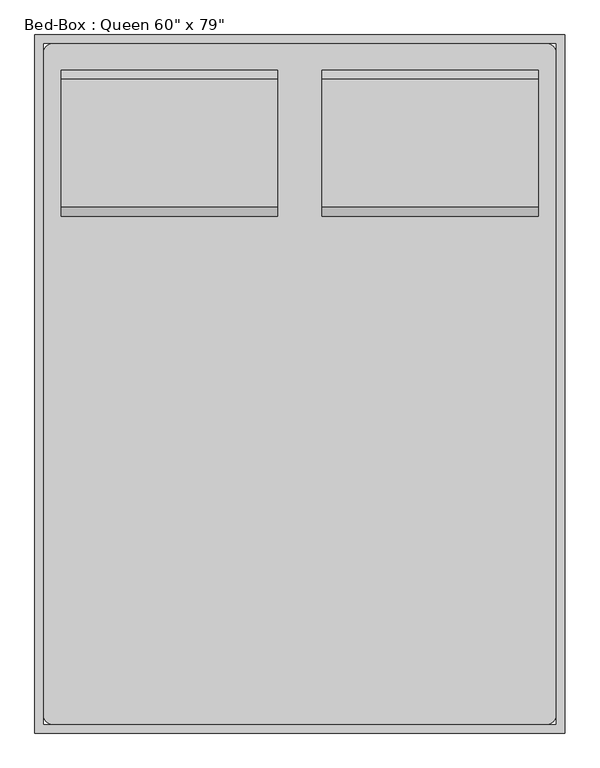
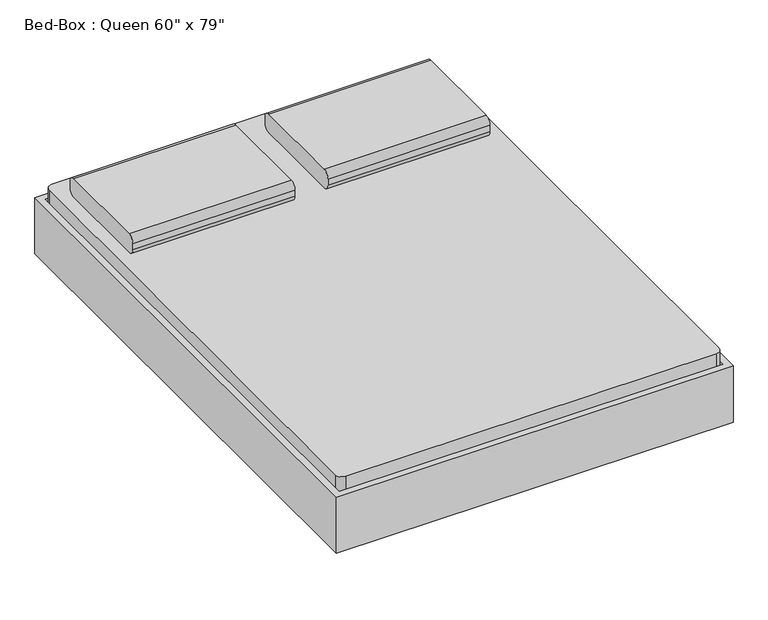
"""IFC4 building model written with IfcOpenShell, lengths in millimetres: furniture geometry."""

from ifc_helpers import new_model, si_unit, point, frame, frame_2d, origin, place, context, project, spatial, polyline, circle_curve, trimmed, segment, composite_curve, outline, extrude, source, transform, mapped, element, save
from ifc_brep_helpers import plane_surface, cylinder_surface, revolved_surface, advanced_brep


def furniture_1d2926bd(model_context):
    return source(origin(), model_context, "Body", "SolidModel", [
        extrude(outline(composite_curve([segment(polyline([(641.8704918, 406.4), (273.5704918, 406.4)]), True, "CONTINUOUS"), segment(trimmed(circle_curve(frame_2d((273.5704918, 431.8)), 25.4), [point((273.5704918, 406.4))], [point((248.1704918, 431.8))], False, "CARTESIAN"), True, "CONTINUOUS"), segment(polyline([(248.1704918, 431.8), (248.1704918, 457.2)]), True, "CONTINUOUS"), segment(trimmed(circle_curve(frame_2d((273.5704918, 457.2)), 25.4), [point((248.1704918, 457.2))], [point((273.5704918, 482.6))], False, "CARTESIAN"), True, "CONTINUOUS"), segment(polyline([(273.5704918, 482.6), (641.8704918, 482.6)]), True, "CONTINUOUS"), segment(trimmed(circle_curve(frame_2d((641.8704918, 457.2)), 25.4), [point((641.8704918, 482.6))], [point((667.2704918, 457.2))], False, "CARTESIAN"), True, "CONTINUOUS"), segment(polyline([(667.2704918, 457.2), (667.2704918, 431.8)]), True, "CONTINUOUS"), segment(trimmed(circle_curve(frame_2d((641.8704918, 431.8)), 25.4), [point((667.2704918, 431.8))], [point((641.8704918, 406.4))], False, "CARTESIAN"), True, "CONTINUOUS")], self_intersect=False)), frame((402.652459, 0.0, 0.0), z_axis=(1.0, 0.0, 0.0), x_axis=(0.0, 1.0, 0.0)), (0.0, 0.0, 1.0), 622.3),
        extrude(outline(composite_curve([segment(polyline([(641.8704918, 406.4), (273.5704918, 406.4)]), True, "CONTINUOUS"), segment(trimmed(circle_curve(frame_2d((273.5704918, 431.8)), 25.4), [point((273.5704918, 406.4))], [point((248.1704918, 431.8))], False, "CARTESIAN"), True, "CONTINUOUS"), segment(polyline([(248.1704918, 431.8), (248.1704918, 457.2)]), True, "CONTINUOUS"), segment(trimmed(circle_curve(frame_2d((273.5704918, 457.2)), 25.4), [point((248.1704918, 457.2))], [point((273.5704918, 482.6))], False, "CARTESIAN"), True, "CONTINUOUS"), segment(polyline([(273.5704918, 482.6), (641.8704918, 482.6)]), True, "CONTINUOUS"), segment(trimmed(circle_curve(frame_2d((641.8704918, 457.2)), 25.4), [point((641.8704918, 482.6))], [point((667.2704918, 457.2))], False, "CARTESIAN"), True, "CONTINUOUS"), segment(polyline([(667.2704918, 457.2), (667.2704918, 431.8)]), True, "CONTINUOUS"), segment(trimmed(circle_curve(frame_2d((641.8704918, 431.8)), 25.4), [point((667.2704918, 431.8))], [point((641.8704918, 406.4))], False, "CARTESIAN"), True, "CONTINUOUS")], self_intersect=False)), frame((-346.647541, 0.0, 0.0), z_axis=(1.0, 0.0, 0.0), x_axis=(0.0, 1.0, 0.0)), (0.0, 0.0, 1.0), 622.3),
        advanced_brep(
        [(-397.1231784, 514.8704918, 177.8), (-397.1231784, 438.6704918, 177.8), (-397.1231784, 438.6704918, 196.85), (-397.1231784, 514.8704918, 196.85), (-346.3231784, 514.8704918, 177.8), (-346.3231784, 438.6704918, 177.8), (-334.1869899, 438.6704918, 196.85), (-334.1869899, 514.8704918, 196.85), (-270.2523099, 514.8704918, 14.6654962), (-270.2523099, 438.6704918, 14.6654962), (-252.9871466, 438.6704918, 22.716374), (-252.9871466, 514.8704918, 22.716374), (-247.2320921, 438.6704918, 0.0), (-247.2320921, 514.8704918, 0.0), (-247.2320921, 438.6704918, 19.05), (-247.2320921, 514.8704918, 19.05), (-168.6195862, 514.8704918, 0.0), (-168.6195862, 438.6704918, 0.0), (-168.6195862, 438.6704918, 19.05), (-168.6195862, 514.8704918, 19.05), (-155.9195862, 438.6704918, 3.4029547), (-155.9195862, 514.8704918, 3.4029547), (-165.4445862, 438.6704918, 19.9007387), (-165.4445862, 514.8704918, 19.9007387), (-95.822541, 514.8704918, 38.1), (-95.822541, 438.6704918, 38.1), (-100.9269731, 438.6704918, 57.15), (-100.9269731, 514.8704918, 57.15), (774.4518216, 514.8704918, 38.1), (774.4518216, 438.6704918, 38.1), (779.5562537, 438.6704918, 57.15), (779.5562537, 514.8704918, 57.15), (834.5488669, 514.8704918, 3.4029547), (834.5488669, 438.6704918, 3.4029547), (844.0738669, 438.6704918, 19.9007387), (844.0738669, 514.8704918, 19.9007387), (847.2488669, 438.6704918, 0.0), (847.2488669, 514.8704918, 0.0), (847.2488669, 438.6704918, 19.05), (847.2488669, 514.8704918, 19.05), (925.8613728, 514.8704918, 0.0), (925.8613728, 438.6704918, 0.0), (925.8613728, 438.6704918, 19.05), (925.8613728, 514.8704918, 19.05), (948.8815906, 438.6704918, 14.6654962), (948.8815906, 514.8704918, 14.6654962), (931.6164272, 438.6704918, 22.716374), (931.6164272, 514.8704918, 22.716374), (1024.952459, 514.8704918, 177.8), (1024.952459, 438.6704918, 177.8), (1012.8162705, 438.6704918, 196.85), (1012.8162705, 514.8704918, 196.85), (1075.752459, 514.8704918, 177.8), (1075.752459, 514.8704918, 196.85), (1075.752459, 438.6704918, 196.85), (1075.752459, 438.6704918, 177.8)],
        [
            (0, 1),
            (1, 2),
            (2, 3),
            (3, 0),
            (0, 4),
            (4, 5),
            (5, 1),
            (5, 6),
            (6, 2),
            (6, 7),
            (7, 3),
            (7, 4),
            (4, 8),
            (8, 9),
            (9, 5),
            (9, 10),
            (10, 6),
            (10, 11),
            (11, 7),
            (11, 8),
            (12, 9, circle_curve(frame((-247.2320921, 438.6704918, 25.4), z_axis=(0.0, 1.0, 0.0), x_axis=(-0.9063077870366486, 0.0, -0.42261826174070233)), 25.4)),
            (8, 13, circle_curve(frame((-247.2320921, 514.8704918, 25.4), z_axis=(0.0, -1.0, 0.0), x_axis=(-0.9063077870366486, 0.0, -0.42261826174070233)), 25.4)),
            (13, 12),
            (14, 10, circle_curve(frame((-247.2320921, 438.6704918, 25.4), z_axis=(0.0, 1.0, 0.0), x_axis=(-0.9063077870366486, 0.0, -0.42261826174070233)), 6.35)),
            (12, 14),
            (15, 11, circle_curve(frame((-247.2320921, 514.8704918, 25.4), z_axis=(0.0, 1.0, 0.0), x_axis=(-0.9063077870366486, 0.0, -0.42261826174070233)), 6.35)),
            (14, 15),
            (15, 13),
            (13, 16),
            (16, 17),
            (17, 12),
            (17, 18),
            (18, 14),
            (18, 19),
            (19, 15),
            (19, 16),
            (20, 17, circle_curve(frame((-168.6195862, 438.6704918, 25.4), z_axis=(0.0, 1.0, 0.0), x_axis=(0.0, 0.0, -1.0)), 25.4)),
            (16, 21, circle_curve(frame((-168.6195862, 514.8704918, 25.4), z_axis=(0.0, -1.0, 0.0), x_axis=(0.0, 0.0, -1.0)), 25.4)),
            (21, 20),
            (22, 18, circle_curve(frame((-168.6195862, 438.6704918, 25.4), z_axis=(0.0, 1.0, 0.0), x_axis=(0.0, 0.0, -1.0)), 6.35)),
            (20, 22),
            (23, 19, circle_curve(frame((-168.6195862, 514.8704918, 25.4), z_axis=(0.0, 1.0, 0.0), x_axis=(0.0, 0.0, -1.0)), 6.35)),
            (22, 23),
            (23, 21),
            (21, 24),
            (24, 25),
            (25, 20),
            (25, 26),
            (26, 22),
            (26, 27),
            (27, 23),
            (27, 24),
            (24, 28),
            (28, 29),
            (29, 25),
            (29, 30),
            (30, 26),
            (30, 31),
            (31, 27),
            (31, 28),
            (28, 32),
            (32, 33),
            (33, 29),
            (33, 34),
            (34, 30),
            (34, 35),
            (35, 31),
            (35, 32),
            (36, 33, circle_curve(frame((847.2488669, 438.6704918, 25.4), z_axis=(0.0, 1.0, 0.0), x_axis=(-0.5000000000000463, 0.0, -0.8660254037844118)), 25.4)),
            (32, 37, circle_curve(frame((847.2488669, 514.8704918, 25.4), z_axis=(0.0, -1.0, 0.0), x_axis=(-0.5000000000000463, 0.0, -0.8660254037844118)), 25.4)),
            (37, 36),
            (38, 34, circle_curve(frame((847.2488669, 438.6704918, 25.4), z_axis=(0.0, 1.0, 0.0), x_axis=(-0.5000000000000463, 0.0, -0.8660254037844118)), 6.35)),
            (36, 38),
            (39, 35, circle_curve(frame((847.2488669, 514.8704918, 25.4), z_axis=(0.0, 1.0, 0.0), x_axis=(-0.5000000000000463, 0.0, -0.8660254037844118)), 6.35)),
            (38, 39),
            (39, 37),
            (37, 40),
            (40, 41),
            (41, 36),
            (41, 42),
            (42, 38),
            (42, 43),
            (43, 39),
            (43, 40),
            (44, 41, circle_curve(frame((925.8613728, 438.6704918, 25.4), z_axis=(0.0, 1.0, 0.0), x_axis=(0.0, 0.0, -1.0)), 25.4)),
            (40, 45, circle_curve(frame((925.8613728, 514.8704918, 25.4), z_axis=(0.0, -1.0, 0.0), x_axis=(0.0, 0.0, -1.0)), 25.4)),
            (45, 44),
            (46, 42, circle_curve(frame((925.8613728, 438.6704918, 25.4), z_axis=(0.0, 1.0, 0.0), x_axis=(0.0, 0.0, -1.0)), 6.35)),
            (44, 46),
            (47, 43, circle_curve(frame((925.8613728, 514.8704918, 25.4), z_axis=(0.0, 1.0, 0.0), x_axis=(0.0, 0.0, -1.0)), 6.35)),
            (46, 47),
            (47, 45),
            (45, 48),
            (48, 49),
            (49, 44),
            (49, 50),
            (50, 46),
            (50, 51),
            (51, 47),
            (51, 48),
            (52, 53),
            (53, 54),
            (54, 55),
            (55, 52),
            (48, 52),
            (55, 49),
            (54, 50),
            (53, 51),
        ],
        [
            plane_surface(frame((-397.1231784, 768.8704918, -152.9490627), z_axis=(-1.0, 0.0, 0.0), x_axis=(0.0, 1.0, 0.0))),
            plane_surface(frame((-397.1231784, 514.8704918, 177.8), z_axis=(0.0, 0.0, -1.0), x_axis=(1.0, 0.0, 0.0))),
            plane_surface(frame((-397.1231784, 438.6704918, 177.8), z_axis=(0.0, -1.0, 0.0), x_axis=(1.0, 0.0, 0.0))),
            plane_surface(frame((-397.1231784, 438.6704918, 196.85), z_axis=(0.0, 0.0, 1.0), x_axis=(1.0, 0.0, 0.0))),
            plane_surface(frame((-397.1231784, 514.8704918, 196.85), z_axis=(0.0, 1.0, 0.0), x_axis=(1.0, 0.0, 0.0))),
            plane_surface(frame((-346.3231784, 514.8704918, 177.8), z_axis=(-0.9063077870366485, 0.0, -0.4226182617407027), x_axis=(0.4226182617407027, 0.0, -0.9063077870366485))),
            plane_surface(frame((-346.3231784, 438.6704918, 177.8), z_axis=(0.0, -1.0, 0.0), x_axis=(0.4226182617407025, 0.0, -0.9063077870366486))),
            plane_surface(frame((-334.1869899, 438.6704918, 196.85), z_axis=(0.9063077870366484, 0.0, 0.4226182617407028), x_axis=(0.4226182617407028, 0.0, -0.9063077870366484))),
            plane_surface(frame((-334.1869899, 514.8704918, 196.85), z_axis=(0.0, 1.0, 0.0), x_axis=(0.42261826174070277, 0.0, -0.9063077870366485))),
            cylinder_surface(frame((-247.2320921, 768.8704918, 25.4), z_axis=(0.0, -1.0, 0.0), x_axis=(-0.9063077870366486, 0.0, -0.42261826174070233)), 25.4),
            plane_surface(frame((-247.2320921, 438.6704918, 25.4), z_axis=(0.0, -1.0, 0.0), x_axis=(-0.9063077870366486, 0.0, -0.42261826174070233))),
            revolved_surface(polyline([(-252.9871465476827, 438.6704918, 22.71637403794654), (-252.9871465476827, 514.8704918, 22.71637403794654)]), (-247.2320921, 768.8704918, 25.4), (0.0, -1.0, 0.0)),
            plane_surface(frame((-247.2320921, 514.8704918, 25.4), z_axis=(0.0, 1.0, 0.0), x_axis=(-0.9063077870366486, 0.0, -0.42261826174070233))),
            plane_surface(frame((-247.2320921, 514.8704918, 0.0), z_axis=(0.0, 0.0, -1.0), x_axis=(1.0, 0.0, 0.0))),
            plane_surface(frame((-247.2320921, 438.6704918, 0.0), z_axis=(0.0, -1.0, 0.0), x_axis=(1.0, 0.0, 0.0))),
            plane_surface(frame((-247.2320921, 438.6704918, 19.05), z_axis=(0.0, 0.0, 1.0), x_axis=(1.0, 0.0, 0.0))),
            plane_surface(frame((-247.2320921, 514.8704918, 19.05), z_axis=(0.0, 1.0, 0.0), x_axis=(1.0, 0.0, 0.0))),
            cylinder_surface(frame((-168.6195862, 768.8704918, 25.4), z_axis=(0.0, -1.0, 0.0), x_axis=(0.0, 0.0, -1.0)), 25.4),
            plane_surface(frame((-168.6195862, 438.6704918, 25.4), z_axis=(0.0, -1.0, 0.0), x_axis=(0.0, 0.0, -1.0))),
            revolved_surface(polyline([(-168.6195862, 438.6704918, 19.049999999999997), (-168.6195862, 514.8704918, 19.049999999999997)]), (-168.6195862, 768.8704918, 25.4), (0.0, -1.0, 0.0)),
            plane_surface(frame((-168.6195862, 514.8704918, 25.4), z_axis=(0.0, 1.0, 0.0), x_axis=(0.0, 0.0, -1.0))),
            plane_surface(frame((-155.9195862, 514.8704918, 3.4029547), z_axis=(0.49999999999988004, 0.0, -0.866025403784508), x_axis=(0.866025403784508, 0.0, 0.49999999999988004))),
            plane_surface(frame((-155.9195862, 438.6704918, 3.4029547), z_axis=(0.0, -1.0, 0.0), x_axis=(0.8660254037845078, 0.0, 0.49999999999988026))),
            plane_surface(frame((-165.4445862, 438.6704918, 19.9007387), z_axis=(-0.4999999999998799, 0.0, 0.866025403784508), x_axis=(0.866025403784508, 0.0, 0.4999999999998799))),
            plane_surface(frame((-165.4445862, 514.8704918, 19.9007387), z_axis=(0.0, 1.0, 0.0), x_axis=(0.8660254037845075, 0.0, 0.49999999999988076))),
            plane_surface(frame((-95.822541, 514.8704918, 38.1), z_axis=(0.0, 0.0, -1.0), x_axis=(1.0, 0.0, 0.0))),
            plane_surface(frame((-95.822541, 438.6704918, 38.1), z_axis=(0.0, -1.0, 0.0), x_axis=(1.0, 0.0, 0.0))),
            plane_surface(frame((-100.9269731, 438.6704918, 57.15), z_axis=(0.0, 0.0, 1.0), x_axis=(1.0, 0.0, 0.0))),
            plane_surface(frame((-100.9269731, 514.8704918, 57.15), z_axis=(0.0, 1.0, 0.0), x_axis=(1.0, 0.0, 0.0))),
            plane_surface(frame((774.4518216, 514.8704918, 38.1), z_axis=(-0.5000000000000455, 0.0, -0.8660254037844125), x_axis=(0.8660254037844125, 0.0, -0.5000000000000455))),
            plane_surface(frame((774.4518216, 438.6704918, 38.1), z_axis=(0.0, -1.0, 0.0), x_axis=(0.866025403784412, 0.0, -0.5000000000000463))),
            plane_surface(frame((779.5562537, 438.6704918, 57.15), z_axis=(0.5000000000000466, 0.0, 0.8660254037844117), x_axis=(0.8660254037844117, 0.0, -0.5000000000000466))),
            plane_surface(frame((779.5562537, 514.8704918, 57.15), z_axis=(0.0, 1.0, 0.0), x_axis=(0.8660254037844115, 0.0, -0.5000000000000471))),
            cylinder_surface(frame((847.2488669, 768.8704918, 25.4), z_axis=(0.0, -1.0, 0.0), x_axis=(-0.5000000000000463, 0.0, -0.8660254037844118)), 25.4),
            plane_surface(frame((847.2488669, 438.6704918, 25.4), z_axis=(0.0, -1.0000000000000002, 0.0), x_axis=(-0.5000000000000464, 0.0, -0.866025403784412))),
            revolved_surface(polyline([(844.0738668999998, 438.6704918, 19.90073868596898), (844.0738668999998, 514.8704918, 19.90073868596898)]), (847.2488669, 768.8704918, 25.4), (0.0, -1.0, 0.0)),
            plane_surface(frame((847.2488669, 514.8704918, 25.4), z_axis=(0.0, 1.0000000000000002, 0.0), x_axis=(-0.5000000000000464, 0.0, -0.866025403784412))),
            plane_surface(frame((847.2488669, 514.8704918, 0.0), z_axis=(0.0, 0.0, -1.0), x_axis=(1.0, 0.0, 0.0))),
            plane_surface(frame((847.2488669, 438.6704918, 0.0), z_axis=(0.0, -1.0, 0.0), x_axis=(1.0, 0.0, 0.0))),
            plane_surface(frame((847.2488669, 438.6704918, 19.05), z_axis=(0.0, 0.0, 1.0), x_axis=(1.0, 0.0, 0.0))),
            plane_surface(frame((847.2488669, 514.8704918, 19.05), z_axis=(0.0, 1.0, 0.0), x_axis=(1.0, 0.0, 0.0))),
            cylinder_surface(frame((925.8613728, 768.8704918, 25.4), z_axis=(0.0, -1.0, 0.0), x_axis=(0.0, 0.0, -1.0)), 25.4),
            plane_surface(frame((925.8613728, 438.6704918, 25.4), z_axis=(0.0, -1.0, 0.0), x_axis=(0.0, 0.0, -1.0))),
            revolved_surface(polyline([(925.8613728, 438.6704918, 19.049999999999997), (925.8613728, 514.8704918, 19.049999999999997)]), (925.8613728, 768.8704918, 25.4), (0.0, -1.0, 0.0)),
            plane_surface(frame((925.8613728, 514.8704918, 25.4), z_axis=(0.0, 1.0, 0.0), x_axis=(0.0, 0.0, -1.0))),
            plane_surface(frame((948.8815906, 514.8704918, 14.6654962), z_axis=(0.90630778703668, 0.0, -0.42261826174063505), x_axis=(0.42261826174063505, 0.0, 0.90630778703668))),
            plane_surface(frame((948.8815906, 438.6704918, 14.6654962), z_axis=(0.0, -1.0, 0.0), x_axis=(0.42261826174063566, 0.0, 0.9063077870366797))),
            plane_surface(frame((931.6164272, 438.6704918, 22.716374), z_axis=(-0.9063077870366801, 0.0, 0.42261826174063477), x_axis=(0.42261826174063477, 0.0, 0.9063077870366801))),
            plane_surface(frame((931.6164272, 514.8704918, 22.716374), z_axis=(0.0, 1.0, 0.0), x_axis=(0.4226182617406345, 0.0, 0.9063077870366802))),
            plane_surface(frame((1075.752459, 768.8704918, -152.9490627), z_axis=(1.0, 0.0, 0.0), x_axis=(0.0, 1.0, 0.0))),
            plane_surface(frame((1024.952459, 514.8704918, 177.8), z_axis=(0.0, 0.0, -1.0), x_axis=(1.0, 0.0, 0.0))),
            plane_surface(frame((1024.952459, 438.6704918, 177.8), z_axis=(0.0, -1.0, 0.0), x_axis=(1.0, 0.0, 0.0))),
            plane_surface(frame((1012.8162705, 438.6704918, 196.85), z_axis=(0.0, 0.0, 1.0), x_axis=(1.0, 0.0, 0.0))),
            plane_surface(frame((1012.8162705, 514.8704918, 196.85), z_axis=(0.0, 1.0, 0.0), x_axis=(1.0, 0.0, 0.0))),
        ],
        [
            (0, [[1, 2, 3, 4]]),
            (1, [[-1, 5, 6, 7]]),
            (2, [[-2, -7, 8, 9]]),
            (3, [[-3, -9, 10, 11]]),
            (4, [[-4, -11, 12, -5]]),
            (5, [[-6, 13, 14, 15]]),
            (6, [[-8, -15, 16, 17]]),
            (7, [[-10, -17, 18, 19]]),
            (8, [[-12, -19, 20, -13]]),
            (9, [[21, -14, 22, 23]]),
            (10, [[24, -16, -21, 25]]),
            (11, [[26, -18, -24, 27]]),
            (12, [[-22, -20, -26, 28]]),
            (13, [[-23, 29, 30, 31]]),
            (14, [[-25, -31, 32, 33]]),
            (15, [[-27, -33, 34, 35]]),
            (16, [[-28, -35, 36, -29]]),
            (17, [[37, -30, 38, 39]]),
            (18, [[40, -32, -37, 41]]),
            (19, [[42, -34, -40, 43]]),
            (20, [[-38, -36, -42, 44]]),
            (21, [[-39, 45, 46, 47]]),
            (22, [[-41, -47, 48, 49]]),
            (23, [[-43, -49, 50, 51]]),
            (24, [[-44, -51, 52, -45]]),
            (25, [[-46, 53, 54, 55]]),
            (26, [[-48, -55, 56, 57]]),
            (27, [[-50, -57, 58, 59]]),
            (28, [[-52, -59, 60, -53]]),
            (29, [[-54, 61, 62, 63]]),
            (30, [[-56, -63, 64, 65]]),
            (31, [[-58, -65, 66, 67]]),
            (32, [[-60, -67, 68, -61]]),
            (33, [[69, -62, 70, 71]]),
            (34, [[72, -64, -69, 73]]),
            (35, [[74, -66, -72, 75]]),
            (36, [[-70, -68, -74, 76]]),
            (37, [[-71, 77, 78, 79]]),
            (38, [[-73, -79, 80, 81]]),
            (39, [[-75, -81, 82, 83]]),
            (40, [[-76, -83, 84, -77]]),
            (41, [[85, -78, 86, 87]]),
            (42, [[88, -80, -85, 89]]),
            (43, [[90, -82, -88, 91]]),
            (44, [[-86, -84, -90, 92]]),
            (45, [[-87, 93, 94, 95]]),
            (46, [[-89, -95, 96, 97]]),
            (47, [[-91, -97, 98, 99]]),
            (48, [[-92, -99, 100, -93]]),
            (49, [[101, 102, 103, 104]]),
            (50, [[-94, 105, -104, 106]]),
            (51, [[-96, -106, -103, 107]]),
            (52, [[-98, -107, -102, 108]]),
            (53, [[-100, -108, -101, -105]]),
        ],
    ),
        extrude(outline(composite_curve([segment(polyline([(-372.047541, 743.4704918), (1050.352459, 743.4704918)]), True, "CONTINUOUS"), segment(trimmed(circle_curve(frame_2d((1050.352459, 718.0704918)), 25.4), [point((1050.352459, 743.4704918))], [point((1075.752459, 718.0704918))], False, "CARTESIAN"), True, "CONTINUOUS"), segment(polyline([(1075.752459, 718.0704918), (1075.752459, -1186.9295082)]), True, "CONTINUOUS"), segment(trimmed(circle_curve(frame_2d((1050.352459, -1186.9295082)), 25.4), [point((1075.752459, -1186.9295082))], [point((1050.352459, -1212.3295082))], False, "CARTESIAN"), True, "CONTINUOUS"), segment(polyline([(1050.352459, -1212.3295082), (-372.047541, -1212.3295082)]), True, "CONTINUOUS"), segment(trimmed(circle_curve(frame_2d((-372.047541, -1186.9295082)), 25.4), [point((-372.047541, -1212.3295082))], [point((-397.447541, -1186.9295082))], False, "CARTESIAN"), True, "CONTINUOUS"), segment(polyline([(-397.447541, -1186.9295082), (-397.447541, 718.0704918)]), True, "CONTINUOUS"), segment(trimmed(circle_curve(frame_2d((-372.047541, 718.0704918)), 25.4), [point((-397.447541, 718.0704918))], [point((-372.047541, 743.4704918))], False, "CARTESIAN"), True, "CONTINUOUS")], self_intersect=False)), frame((0.0, 0.0, 203.2), z_axis=(0.0, 0.0, 1.0), x_axis=(1.0, 0.0, 0.0)), (0.0, 0.0, 1.0), 203.2),
        advanced_brep(
        [(-397.447541, -932.9295082, 196.85), (-397.447541, -932.9295082, 177.8), (-397.447541, -1009.1295082, 177.8), (-397.447541, -1009.1295082, 196.85), (-334.5113525, -932.9295082, 196.85), (-346.647541, -932.9295082, 177.8), (-346.647541, -1009.1295082, 177.8), (-334.5113525, -1009.1295082, 196.85), (-253.3115092, -932.9295082, 22.716374), (-270.5766725, -932.9295082, 14.6654962), (-270.5766725, -1009.1295082, 14.6654962), (-253.3115092, -1009.1295082, 22.716374), (-247.5564547, -932.9295082, 0.0), (-247.5564547, -932.9295082, 19.05), (-247.5564547, -1009.1295082, 0.0), (-247.5564547, -1009.1295082, 19.05), (-168.9439489, -932.9295082, 19.05), (-168.9439489, -932.9295082, 0.0), (-168.9439489, -1009.1295082, 0.0), (-168.9439489, -1009.1295082, 19.05), (-156.2439489, -932.9295082, 3.4029547), (-165.7689489, -932.9295082, 19.9007387), (-156.2439489, -1009.1295082, 3.4029547), (-165.7689489, -1009.1295082, 19.9007387), (-101.2513357, -932.9295082, 57.15), (-96.1469036, -932.9295082, 38.1), (-96.1469036, -1009.1295082, 38.1), (-101.2513357, -1009.1295082, 57.15), (779.5562537, -932.9295082, 57.15), (774.4518216, -932.9295082, 38.1), (774.4518216, -1009.1295082, 38.1), (779.5562537, -1009.1295082, 57.15), (844.0738669, -932.9295082, 19.9007387), (834.5488669, -932.9295082, 3.4029547), (834.5488669, -1009.1295082, 3.4029547), (844.0738669, -1009.1295082, 19.9007387), (847.2488669, -932.9295082, 0.0), (847.2488669, -932.9295082, 19.05), (847.2488669, -1009.1295082, 0.0), (847.2488669, -1009.1295082, 19.05), (925.8613728, -932.9295082, 19.05), (925.8613728, -932.9295082, 0.0), (925.8613728, -1009.1295082, 0.0), (925.8613728, -1009.1295082, 19.05), (948.8815906, -932.9295082, 14.6654962), (931.6164272, -932.9295082, 22.716374), (948.8815906, -1009.1295082, 14.6654962), (931.6164272, -1009.1295082, 22.716374), (1012.8162705, -932.9295082, 196.85), (1024.952459, -932.9295082, 177.8), (1024.952459, -1009.1295082, 177.8), (1012.8162705, -1009.1295082, 196.85), (1075.752459, -932.9295082, 196.85), (1075.752459, -1009.1295082, 196.85), (1075.752459, -1009.1295082, 177.8), (1075.752459, -932.9295082, 177.8)],
        [
            (0, 1),
            (1, 2),
            (2, 3),
            (3, 0),
            (0, 4),
            (4, 5),
            (5, 1),
            (5, 6),
            (6, 2),
            (6, 7),
            (7, 3),
            (7, 4),
            (4, 8),
            (8, 9),
            (9, 5),
            (9, 10),
            (10, 6),
            (10, 11),
            (11, 7),
            (11, 8),
            (12, 9, circle_curve(frame((-247.5564547, -932.9295082, 25.4), z_axis=(0.0, 1.0, 0.0), x_axis=(-0.906307787036663, 0.0, -0.4226182617406713)), 25.4)),
            (8, 13, circle_curve(frame((-247.5564547, -932.9295082, 25.4), z_axis=(0.0, -1.0, 0.0), x_axis=(-0.906307787036663, 0.0, -0.4226182617406713)), 6.35)),
            (13, 12),
            (14, 10, circle_curve(frame((-247.5564547, -1009.1295082, 25.4), z_axis=(0.0, 1.0, 0.0), x_axis=(-0.906307787036663, 0.0, -0.4226182617406713)), 25.4)),
            (12, 14),
            (15, 11, circle_curve(frame((-247.5564547, -1009.1295082, 25.4), z_axis=(0.0, 1.0, 0.0), x_axis=(-0.906307787036663, 0.0, -0.4226182617406713)), 6.35)),
            (14, 15),
            (15, 13),
            (13, 16),
            (16, 17),
            (17, 12),
            (17, 18),
            (18, 14),
            (18, 19),
            (19, 15),
            (19, 16),
            (20, 17, circle_curve(frame((-168.9439489, -932.9295082, 25.4), z_axis=(0.0, 1.0, 0.0), x_axis=(0.0, 0.0, -1.0)), 25.4)),
            (16, 21, circle_curve(frame((-168.9439489, -932.9295082, 25.4), z_axis=(0.0, -1.0, 0.0), x_axis=(0.0, 0.0, -1.0)), 6.35)),
            (21, 20),
            (22, 18, circle_curve(frame((-168.9439489, -1009.1295082, 25.4), z_axis=(0.0, 1.0, 0.0), x_axis=(0.0, 0.0, -1.0)), 25.4)),
            (20, 22),
            (23, 19, circle_curve(frame((-168.9439489, -1009.1295082, 25.4), z_axis=(0.0, 1.0, 0.0), x_axis=(0.0, 0.0, -1.0)), 6.35)),
            (22, 23),
            (23, 21),
            (21, 24),
            (24, 25),
            (25, 20),
            (25, 26),
            (26, 22),
            (26, 27),
            (27, 23),
            (27, 24),
            (24, 28),
            (28, 29),
            (29, 25),
            (29, 30),
            (30, 26),
            (30, 31),
            (31, 27),
            (31, 28),
            (28, 32),
            (32, 33),
            (33, 29),
            (33, 34),
            (34, 30),
            (34, 35),
            (35, 31),
            (35, 32),
            (36, 33, circle_curve(frame((847.2488669, -932.9295082, 25.4), z_axis=(0.0, 1.0, 0.0), x_axis=(-0.5000000000000479, 0.0, -0.866025403784411)), 25.4)),
            (32, 37, circle_curve(frame((847.2488669, -932.9295082, 25.4), z_axis=(0.0, -1.0, 0.0), x_axis=(-0.5000000000000479, 0.0, -0.866025403784411)), 6.35)),
            (37, 36),
            (38, 34, circle_curve(frame((847.2488669, -1009.1295082, 25.4), z_axis=(0.0, 1.0, 0.0), x_axis=(-0.5000000000000479, 0.0, -0.866025403784411)), 25.4)),
            (36, 38),
            (39, 35, circle_curve(frame((847.2488669, -1009.1295082, 25.4), z_axis=(0.0, 1.0, 0.0), x_axis=(-0.5000000000000479, 0.0, -0.866025403784411)), 6.35)),
            (38, 39),
            (39, 37),
            (37, 40),
            (40, 41),
            (41, 36),
            (41, 42),
            (42, 38),
            (42, 43),
            (43, 39),
            (43, 40),
            (44, 41, circle_curve(frame((925.8613728, -932.9295082, 25.4), z_axis=(0.0, 1.0, 0.0), x_axis=(0.0, 0.0, -1.0)), 25.4)),
            (40, 45, circle_curve(frame((925.8613728, -932.9295082, 25.4), z_axis=(0.0, -1.0, 0.0), x_axis=(0.0, 0.0, -1.0)), 6.35)),
            (45, 44),
            (46, 42, circle_curve(frame((925.8613728, -1009.1295082, 25.4), z_axis=(0.0, 1.0, 0.0), x_axis=(0.0, 0.0, -1.0)), 25.4)),
            (44, 46),
            (47, 43, circle_curve(frame((925.8613728, -1009.1295082, 25.4), z_axis=(0.0, 1.0, 0.0), x_axis=(0.0, 0.0, -1.0)), 6.35)),
            (46, 47),
            (47, 45),
            (45, 48),
            (48, 49),
            (49, 44),
            (49, 50),
            (50, 46),
            (50, 51),
            (51, 47),
            (51, 48),
            (52, 53),
            (53, 54),
            (54, 55),
            (55, 52),
            (48, 52),
            (55, 49),
            (54, 50),
            (53, 51),
        ],
        [
            plane_surface(frame((-397.447541, -1237.7295082, -127.5947323), z_axis=(-1.0, 0.0, 0.0), x_axis=(0.0, 1.0, 0.0))),
            plane_surface(frame((-397.447541, -932.9295082, 196.85), z_axis=(0.0, 1.0, 0.0), x_axis=(1.0, 0.0, 0.0))),
            plane_surface(frame((-397.447541, -932.9295082, 177.8), z_axis=(0.0, 0.0, -1.0), x_axis=(1.0, 0.0, 0.0))),
            plane_surface(frame((-397.447541, -1009.1295082, 177.8), z_axis=(0.0, -1.0, 0.0), x_axis=(1.0, 0.0, 0.0))),
            plane_surface(frame((-397.447541, -1009.1295082, 196.85), z_axis=(0.0, 0.0, 1.0), x_axis=(1.0, 0.0, 0.0))),
            plane_surface(frame((-334.5113525, -932.9295082, 196.85), z_axis=(0.0, 1.0, 0.0), x_axis=(0.4226182617406707, 0.0, -0.9063077870366634))),
            plane_surface(frame((-346.647541, -932.9295082, 177.8), z_axis=(-0.9063077870366635, 0.0, -0.4226182617406707), x_axis=(0.4226182617406707, 0.0, -0.9063077870366635))),
            plane_surface(frame((-346.647541, -1009.1295082, 177.8), z_axis=(0.0, -1.0, 0.0), x_axis=(0.422618261740671, 0.0, -0.9063077870366633))),
            plane_surface(frame((-334.5113525, -1009.1295082, 196.85), z_axis=(0.9063077870366633, 0.0, 0.42261826174067113), x_axis=(0.42261826174067113, 0.0, -0.9063077870366633))),
            plane_surface(frame((-247.5564547, -932.9295082, 25.4), z_axis=(0.0, 1.0, 0.0), x_axis=(-0.906307787036663, 0.0, -0.4226182617406713))),
            cylinder_surface(frame((-247.5564547, -1237.7295082, 25.4), z_axis=(0.0, -1.0, 0.0), x_axis=(-0.906307787036663, 0.0, -0.4226182617406713)), 25.4),
            plane_surface(frame((-247.5564547, -1009.1295082, 25.4), z_axis=(0.0, -1.0, 0.0), x_axis=(-0.906307787036663, 0.0, -0.4226182617406713))),
            revolved_surface(polyline([(-253.3115091476828, -1009.1295082, 22.716374037946736), (-253.3115091476828, -932.9295082, 22.716374037946736)]), (-247.5564547, -1237.7295082, 25.4), (0.0, -1.0, 0.0)),
            plane_surface(frame((-247.5564547, -932.9295082, 19.05), z_axis=(0.0, 1.0, 0.0), x_axis=(1.0, 0.0, 0.0))),
            plane_surface(frame((-247.5564547, -932.9295082, 0.0), z_axis=(0.0, 0.0, -1.0), x_axis=(1.0, 0.0, 0.0))),
            plane_surface(frame((-247.5564547, -1009.1295082, 0.0), z_axis=(0.0, -1.0, 0.0), x_axis=(1.0, 0.0, 0.0))),
            plane_surface(frame((-247.5564547, -1009.1295082, 19.05), z_axis=(0.0, 0.0, 1.0), x_axis=(1.0, 0.0, 0.0))),
            plane_surface(frame((-168.9439489, -932.9295082, 25.4), z_axis=(0.0, 1.0, 0.0), x_axis=(0.0, 0.0, -1.0))),
            cylinder_surface(frame((-168.9439489, -1237.7295082, 25.4), z_axis=(0.0, -1.0, 0.0), x_axis=(0.0, 0.0, -1.0)), 25.4),
            plane_surface(frame((-168.9439489, -1009.1295082, 25.4), z_axis=(0.0, -1.0, 0.0), x_axis=(0.0, 0.0, -1.0))),
            revolved_surface(polyline([(-168.9439489, -1009.1295082, 19.049999999999997), (-168.9439489, -932.9295082, 19.049999999999997)]), (-168.9439489, -1237.7295082, 25.4), (0.0, -1.0, 0.0)),
            plane_surface(frame((-165.7689489, -932.9295082, 19.9007387), z_axis=(0.0, 1.0, 0.0), x_axis=(0.8660254037844788, 0.0, 0.4999999999999306))),
            plane_surface(frame((-156.2439489, -932.9295082, 3.4029547), z_axis=(0.49999999999993017, 0.0, -0.866025403784479), x_axis=(0.866025403784479, 0.0, 0.49999999999993017))),
            plane_surface(frame((-156.2439489, -1009.1295082, 3.4029547), z_axis=(0.0, -1.0, 0.0), x_axis=(0.8660254037844785, 0.0, 0.49999999999993106))),
            plane_surface(frame((-165.7689489, -1009.1295082, 19.9007387), z_axis=(-0.4999999999999309, 0.0, 0.8660254037844786), x_axis=(0.8660254037844786, 0.0, 0.4999999999999309))),
            plane_surface(frame((-101.2513357, -932.9295082, 57.15), z_axis=(0.0, 1.0, 0.0), x_axis=(1.0, 0.0, 0.0))),
            plane_surface(frame((-96.1469036, -932.9295082, 38.1), z_axis=(0.0, 0.0, -1.0), x_axis=(1.0, 0.0, 0.0))),
            plane_surface(frame((-96.1469036, -1009.1295082, 38.1), z_axis=(0.0, -1.0, 0.0), x_axis=(1.0, 0.0, 0.0))),
            plane_surface(frame((-101.2513357, -1009.1295082, 57.15), z_axis=(0.0, 0.0, 1.0), x_axis=(1.0, 0.0, 0.0))),
            plane_surface(frame((779.5562537, -932.9295082, 57.15), z_axis=(0.0, 1.0000000000000002, 0.0), x_axis=(0.8660254037844106, 0.0, -0.5000000000000487))),
            plane_surface(frame((774.4518216, -932.9295082, 38.1), z_axis=(-0.5000000000000477, 0.0, -0.8660254037844112), x_axis=(0.8660254037844112, 0.0, -0.5000000000000477))),
            plane_surface(frame((774.4518216, -1009.1295082, 38.1), z_axis=(0.0, -1.0000000000000002, 0.0), x_axis=(0.8660254037844105, 0.0, -0.500000000000049))),
            plane_surface(frame((779.5562537, -1009.1295082, 57.15), z_axis=(0.5000000000000498, 0.0, 0.8660254037844098), x_axis=(0.8660254037844098, 0.0, -0.5000000000000498))),
            plane_surface(frame((847.2488669, -932.9295082, 25.4), z_axis=(0.0, 1.0000000000000002, 0.0), x_axis=(-0.500000000000048, 0.0, -0.8660254037844111))),
            cylinder_surface(frame((847.2488669, -1237.7295082, 25.4), z_axis=(0.0, -1.0, 0.0), x_axis=(-0.5000000000000479, 0.0, -0.866025403784411)), 25.4),
            plane_surface(frame((847.2488669, -1009.1295082, 25.4), z_axis=(0.0, -1.0000000000000002, 0.0), x_axis=(-0.500000000000048, 0.0, -0.8660254037844111))),
            revolved_surface(polyline([(844.0738668999998, -1009.1295082, 19.90073868596899), (844.0738668999998, -932.9295082, 19.90073868596899)]), (847.2488669, -1237.7295082, 25.4), (0.0, -1.0, 0.0)),
            plane_surface(frame((847.2488669, -932.9295082, 19.05), z_axis=(0.0, 1.0, 0.0), x_axis=(1.0, 0.0, 0.0))),
            plane_surface(frame((847.2488669, -932.9295082, 0.0), z_axis=(0.0, 0.0, -1.0), x_axis=(1.0, 0.0, 0.0))),
            plane_surface(frame((847.2488669, -1009.1295082, 0.0), z_axis=(0.0, -1.0, 0.0), x_axis=(1.0, 0.0, 0.0))),
            plane_surface(frame((847.2488669, -1009.1295082, 19.05), z_axis=(0.0, 0.0, 1.0), x_axis=(1.0, 0.0, 0.0))),
            plane_surface(frame((925.8613728, -932.9295082, 25.4), z_axis=(0.0, 1.0, 0.0), x_axis=(0.0, 0.0, -1.0))),
            cylinder_surface(frame((925.8613728, -1237.7295082, 25.4), z_axis=(0.0, -1.0, 0.0), x_axis=(0.0, 0.0, -1.0)), 25.4),
            plane_surface(frame((925.8613728, -1009.1295082, 25.4), z_axis=(0.0, -1.0, 0.0), x_axis=(0.0, 0.0, -1.0))),
            revolved_surface(polyline([(925.8613728, -1009.1295082, 19.049999999999997), (925.8613728, -932.9295082, 19.049999999999997)]), (925.8613728, -1237.7295082, 25.4), (0.0, -1.0, 0.0)),
            plane_surface(frame((931.6164272, -932.9295082, 22.716374), z_axis=(0.0, 1.0, 0.0), x_axis=(0.4226182617405411, 0.0, 0.9063077870367238))),
            plane_surface(frame((948.8815906, -932.9295082, 14.6654962), z_axis=(0.9063077870367237, 0.0, -0.4226182617405414), x_axis=(0.4226182617405414, 0.0, 0.9063077870367237))),
            plane_surface(frame((948.8815906, -1009.1295082, 14.6654962), z_axis=(0.0, -1.0, 0.0), x_axis=(0.42261826174054123, 0.0, 0.9063077870367238))),
            plane_surface(frame((931.6164272, -1009.1295082, 22.716374), z_axis=(-0.9063077870367237, 0.0, 0.4226182617405414), x_axis=(0.4226182617405414, 0.0, 0.9063077870367237))),
            plane_surface(frame((1075.752459, -1237.7295082, -127.5947323), z_axis=(1.0, 0.0, 0.0), x_axis=(0.0, 1.0, 0.0))),
            plane_surface(frame((1012.8162705, -932.9295082, 196.85), z_axis=(0.0, 1.0, 0.0), x_axis=(1.0, 0.0, 0.0))),
            plane_surface(frame((1024.952459, -932.9295082, 177.8), z_axis=(0.0, 0.0, -1.0), x_axis=(1.0, 0.0, 0.0))),
            plane_surface(frame((1024.952459, -1009.1295082, 177.8), z_axis=(0.0, -1.0, 0.0), x_axis=(1.0, 0.0, 0.0))),
            plane_surface(frame((1012.8162705, -1009.1295082, 196.85), z_axis=(0.0, 0.0, 1.0), x_axis=(1.0, 0.0, 0.0))),
        ],
        [
            (0, [[1, 2, 3, 4]]),
            (1, [[-1, 5, 6, 7]]),
            (2, [[-2, -7, 8, 9]]),
            (3, [[-3, -9, 10, 11]]),
            (4, [[-4, -11, 12, -5]]),
            (5, [[-6, 13, 14, 15]]),
            (6, [[-8, -15, 16, 17]]),
            (7, [[-10, -17, 18, 19]]),
            (8, [[-12, -19, 20, -13]]),
            (9, [[21, -14, 22, 23]]),
            (10, [[24, -16, -21, 25]]),
            (11, [[26, -18, -24, 27]]),
            (12, [[-22, -20, -26, 28]]),
            (13, [[-23, 29, 30, 31]]),
            (14, [[-25, -31, 32, 33]]),
            (15, [[-27, -33, 34, 35]]),
            (16, [[-28, -35, 36, -29]]),
            (17, [[37, -30, 38, 39]]),
            (18, [[40, -32, -37, 41]]),
            (19, [[42, -34, -40, 43]]),
            (20, [[-38, -36, -42, 44]]),
            (21, [[-39, 45, 46, 47]]),
            (22, [[-41, -47, 48, 49]]),
            (23, [[-43, -49, 50, 51]]),
            (24, [[-44, -51, 52, -45]]),
            (25, [[-46, 53, 54, 55]]),
            (26, [[-48, -55, 56, 57]]),
            (27, [[-50, -57, 58, 59]]),
            (28, [[-52, -59, 60, -53]]),
            (29, [[-54, 61, 62, 63]]),
            (30, [[-56, -63, 64, 65]]),
            (31, [[-58, -65, 66, 67]]),
            (32, [[-60, -67, 68, -61]]),
            (33, [[69, -62, 70, 71]]),
            (34, [[72, -64, -69, 73]]),
            (35, [[74, -66, -72, 75]]),
            (36, [[-70, -68, -74, 76]]),
            (37, [[-71, 77, 78, 79]]),
            (38, [[-73, -79, 80, 81]]),
            (39, [[-75, -81, 82, 83]]),
            (40, [[-76, -83, 84, -77]]),
            (41, [[85, -78, 86, 87]]),
            (42, [[88, -80, -85, 89]]),
            (43, [[90, -82, -88, 91]]),
            (44, [[-86, -84, -90, 92]]),
            (45, [[-87, 93, 94, 95]]),
            (46, [[-89, -95, 96, 97]]),
            (47, [[-91, -97, 98, 99]]),
            (48, [[-92, -99, 100, -93]]),
            (49, [[101, 102, 103, 104]]),
            (50, [[-94, 105, -104, 106]]),
            (51, [[-96, -106, -103, 107]]),
            (52, [[-98, -107, -102, 108]]),
            (53, [[-100, -108, -101, -105]]),
        ],
    ),
        extrude(outline(polyline([(1101.152459, 768.8704918), (1101.152459, -1237.7295082), (-422.847541, -1237.7295082), (-422.847541, 768.8704918), (1101.152459, 768.8704918)]), holes=[polyline([(1075.752459, 743.4704918), (-397.447541, 743.4704918), (-397.447541, -1212.3295082), (1075.752459, -1212.3295082), (1075.752459, 743.4704918)])]), frame((0.0, 0.0, 127.0), z_axis=(0.0, 0.0, 1.0), x_axis=(1.0, 0.0, 0.0)), (0.0, 0.0, 1.0), 228.6),
    ])


if __name__ == "__main__":
    model = new_model("IFC4")
    model_context = context("Model", 3, world=origin())
    ifc_project = project(units=[si_unit("LENGTHUNIT", "METRE", prefix="MILLI")], contexts=[model_context])
    site = spatial("IfcSite", under=ifc_project)
    building = spatial("IfcBuilding", under=site)
    placement = place(None, origin())
    furniture_shape = furniture_1d2926bd(model_context)
    element("IfcFurniture", 1, ObjectType="Bed-Box : Queen 60\" x 79\"", at=placement, inside=building, context=model_context, shape_type="MappedRepresentation", body=[
        mapped(furniture_shape, transform((0.0, 0.0, 0.0), x_axis=(1.0, 0.0, 0.0), y_axis=(0.0, 1.0, 0.0), z_axis=(0.0, 0.0, 1.0))),
    ])
    save(model, "model.ifc")

# Revit data of these elements
# Type "Bed-Box : Queen 60\" x 79\""
#   Assembly Code = "E2020200"
#   Length = 6' - 7"
#   Width = 5' - 0"
#   Frame Material = Birch
#   Mattress Material = Sash
#   Default Elevation = 0
# Element 1 (IfcFurniture, "Bed-Box : Queen 60\" x 79\"")
#   Materials on its faces: "Birch", "Sash"
# Materials
#   "Birch": class "Wood", colour RGB 210 159 95, transparency 0, Description = "Betula Alleghaniensis", Cost = 0
#   "Sash": class "Wood", colour RGB 224 178 126, transparency 0
